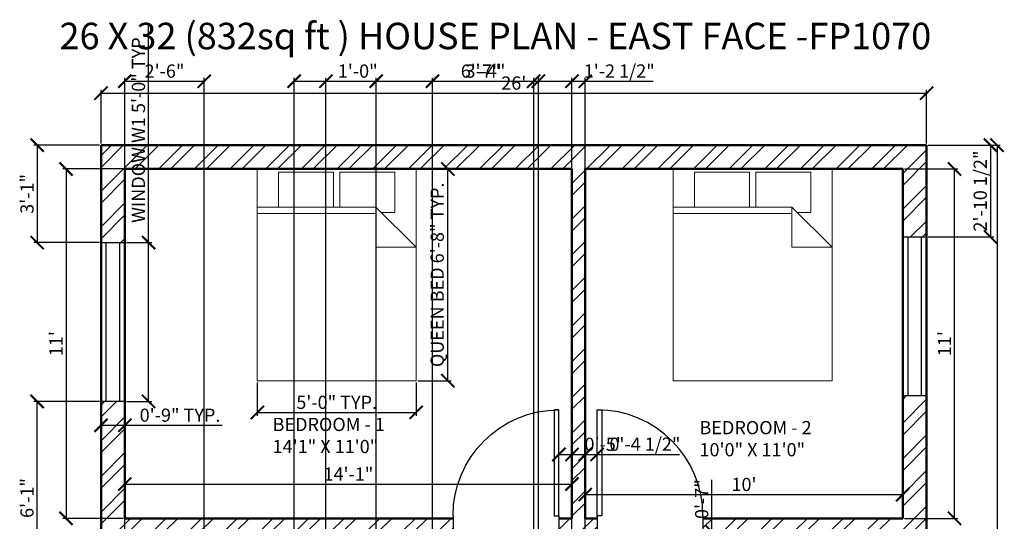
# Model space of a CAD drawing. Units: inches. Extents: x 683 to 1274, y 1901 to 2385.
# Tile 4 of 5: x 687 to 1059, y 2196 to 2385. Entities that reach past the tile are written whole.
import ezdxf

# ---------------------------------------------------------------- set-up
doc = ezdxf.new("R2010")
doc.units = ezdxf.units.IN
for name, color, linetype, lineweight in [('A-AREA-IDEN', 3, 'Continuous', 25), ('A-FURN', 2, 'Continuous', 18), ('A-WALL-PATT', 8, 'Continuous', 13), ('DIM', 3, 'Continuous', 18), ('DOORS', 4, 'Continuous', 25), ('TEXT', 1, 'Continuous', 25), ('walls', 6, 'Continuous', 50), ('WINDOWS', 30, 'Continuous', 25)]:
    doc.layers.add(name, color=color, linetype=linetype, lineweight=lineweight)
doc.styles.get("Standard").update_dxf_attribs({"font": 'arial.ttf'})
doc.dimstyles.new('ISO-25', dxfattribs={"dimtxt": 5, "dimasz": 5, "dimexe": 1.25, "dimexo": 0.625, "dimtad": 1, "dimdec": 1, "dimlunit": 4, "dimtxsty": 'Standard', "dimblk": 'ARCHTICK', "dimcen": 2.5, "dimadec": 0, "dimazin": 0, "dimtfac": 1, "dimtdec": 1, "dimtmove": 0, "dimatfit": 3, "dimfxl": 1, "dimarcsym": 0})

# ---------------------------------------------------------------- blocks, each defined once
blk = doc.blocks.new('Bed - Queen')
for p, q in [((0, -80.00003), (0, 0)), ((0, 0), (59.99999, 0)), ((59.99999, 0), (59.99999, -80.00003)), ((7.99999, -1.2), (28.79998, -1.2)), ((7.99999, -14.4), (7.99999, -1.2)), ((28.79998, -1.2), (28.79998, -14.4)), ((31.19999, -1.2), (51.99999, -1.2)), ((31.19999, -14.4), (31.19999, -1.2)), ((51.99999, -1.2), (51.99999, -16.4)), ((0, -14.4), (44.8, -14.4)), ((59.99999, -29.6), (44.8, -14.4)), ((44.8, -14.4), (44.8, -29.6)), ((44.8, -16.8), (0, -16.8)), ((51.99999, -16.4), (46.79936, -16.4)), ((44.8, -29.6), (59.99999, -29.6)), ((59.99999, -80.00003), (0, -80.00003))]:
    blk.add_line(p, q)
blk = doc.blocks.new('_ArchTick')
at = {"color": 0, "linetype": 'ByBlock', "const_width": 0.15}
blk.add_lwpolyline([(-0.5, -0.5), (0.5, 0.5)], dxfattribs=at)
blk = doc.blocks.new('*D6')
at = {"layer": 'Defpoints', "color": 0, "transparency": 16777216}
for p in [(1029.42, 2357.4), (717.42, 2337.78), (1029.42, 2337.78)]:
    blk.add_point(p, dxfattribs=at)
at = {"layer": 'DIM', "color": 0, "lineweight": -2, "transparency": 16777216}
for p, q in [((717.42, 2338.41), (717.42, 2358.65)), ((717.42, 2357.4), (1029.42, 2357.4)), ((1029.42, 2338.41), (1029.42, 2358.65))]:
    blk.add_line(p, q, dxfattribs=at)
at = {"layer": 'DIM', "color": 0, "lineweight": -2, "transparency": 16777216, "xscale": 5, "yscale": 5, "zscale": 5, "rotation": 180}
blk.add_blockref('_ArchTick', (717.42, 2357.4), dxfattribs=at)
at = {"layer": 'DIM', "color": 0, "lineweight": -2, "transparency": 16777216, "xscale": 5, "yscale": 5, "zscale": 5}
blk.add_blockref('_ArchTick', (1029.42, 2357.4), dxfattribs=at)
at = {"layer": 'DIM', "color": 0, "transparency": 16777216, "insert": (873.42, 2360.58), "char_height": 5, "attachment_point": 5}
blk.add_mtext("26'", dxfattribs=at)
blk = doc.blocks.new('*D7')
at = {"layer": 'Defpoints', "color": 0, "transparency": 16777216}
for p in [(1029.42, 2337.78), (1029.42, 1953.78), (1056.05, 1953.78)]:
    blk.add_point(p, dxfattribs=at)
at = {"layer": 'DIM', "color": 0, "lineweight": -2, "transparency": 16777216}
for p, q in [((1030.04, 2337.78), (1057.3, 2337.78)), ((1056.05, 2337.78), (1056.05, 1953.78)), ((1030.04, 1953.78), (1057.3, 1953.78))]:
    blk.add_line(p, q, dxfattribs=at)
at = {"layer": 'DIM', "color": 0, "lineweight": -2, "transparency": 16777216, "xscale": 5, "yscale": 5, "zscale": 5}
for p, rotation in [((1056.05, 2337.78), 90), ((1056.05, 1953.78), 270)]:
    blk.add_blockref('_ArchTick', p, dxfattribs=dict(at, rotation=rotation))
at = {"layer": 'DIM', "color": 0, "transparency": 16777216, "insert": (1052.87, 2145.78), "char_height": 5, "attachment_point": 5, "rotation": 90}
blk.add_mtext("32'", dxfattribs=at)
blk = doc.blocks.new('*D9')
at = {"layer": 'Defpoints', "color": 0, "transparency": 16777216}
for p in [(895.42, 2209.73), (726.42, 2196.78), (895.42, 2196.78)]:
    blk.add_point(p, dxfattribs=at)
at = {"layer": 'DIM', "color": 0, "lineweight": -2, "transparency": 16777216}
for p, q in [((726.42, 2197.41), (726.42, 2210.98)), ((895.42, 2197.41), (895.42, 2210.98)), ((726.42, 2209.73), (895.42, 2209.73))]:
    blk.add_line(p, q, dxfattribs=at)
at = {"layer": 'DIM', "color": 0, "lineweight": -2, "transparency": 16777216, "xscale": 5, "yscale": 5, "zscale": 5, "rotation": 180}
blk.add_blockref('_ArchTick', (726.42, 2209.73), dxfattribs=at)
at = {"layer": 'DIM', "color": 0, "lineweight": -2, "transparency": 16777216, "xscale": 5, "yscale": 5, "zscale": 5}
blk.add_blockref('_ArchTick', (895.42, 2209.73), dxfattribs=at)
at = {"layer": 'DIM', "color": 0, "transparency": 16777216, "insert": (810.92, 2212.86), "char_height": 5, "attachment_point": 5}
blk.add_mtext('14\'-1"', dxfattribs=at)
blk = doc.blocks.new('*D10')
at = {"layer": 'Defpoints', "color": 0, "transparency": 16777216}
for p in [(1020.42, 2205.76), (900.42, 2196.78), (1020.42, 2196.78)]:
    blk.add_point(p, dxfattribs=at)
at = {"layer": 'DIM', "color": 0, "lineweight": -2, "transparency": 16777216}
for p, q in [((900.42, 2197.41), (900.42, 2207.01)), ((1020.42, 2197.41), (1020.42, 2207.01)), ((900.42, 2205.76), (1020.42, 2205.76))]:
    blk.add_line(p, q, dxfattribs=at)
at = {"layer": 'DIM', "color": 0, "lineweight": -2, "transparency": 16777216, "xscale": 5, "yscale": 5, "zscale": 5, "rotation": 180}
blk.add_blockref('_ArchTick', (900.42, 2205.76), dxfattribs=at)
at = {"layer": 'DIM', "color": 0, "lineweight": -2, "transparency": 16777216, "xscale": 5, "yscale": 5, "zscale": 5}
blk.add_blockref('_ArchTick', (1020.42, 2205.76), dxfattribs=at)
at = {"layer": 'DIM', "color": 0, "transparency": 16777216, "insert": (960.42, 2208.94), "char_height": 5, "attachment_point": 5}
blk.add_mtext("10'", dxfattribs=at)
blk = doc.blocks.new('W1')
at = {"layer": 'WINDOWS'}
for p, q in [((1078.63, 2170.04), (1087.63, 2170.04)), ((1078.63, 2110.04), (1078.63, 2170.04)), ((1080.63, 2110.04), (1080.63, 2170.04)), ((1085.63, 2170.04), (1085.63, 2110.04)), ((1087.63, 2170.04), (1087.63, 2110.04)), ((1087.63, 2110.04), (1078.63, 2110.04))]:
    blk.add_line(p, q, dxfattribs=at)
blk = doc.blocks.new('*U18')
for p, q in [((0, 0), (0, -6)), ((40, 0), (40, -6))]:
    blk.add_line(p, q)
blk.add_lwpolyline([(0, 0), (0, 40), (1.75, 40), (1.75, 0)], close=True)
blk.add_arc((0, 0), 40, 0, 90)
blk = doc.blocks.new('*D19')
at = {"layer": 'Defpoints', "color": 0, "transparency": 16777216}
for p in [(726.42, 2328.78), (704.19, 2196.78), (726.42, 2196.78)]:
    blk.add_point(p, dxfattribs=at)
at = {"layer": 'DIM', "color": 0, "lineweight": -2, "transparency": 16777216}
for p, q in [((725.79, 2328.78), (702.94, 2328.78)), ((704.19, 2328.78), (704.19, 2196.78)), ((725.79, 2196.78), (702.94, 2196.78))]:
    blk.add_line(p, q, dxfattribs=at)
at = {"layer": 'DIM', "color": 0, "lineweight": -2, "transparency": 16777216, "xscale": 5, "yscale": 5, "zscale": 5}
for p, rotation in [((704.19, 2328.78), 90), ((704.19, 2196.78), 270)]:
    blk.add_blockref('_ArchTick', p, dxfattribs=dict(at, rotation=rotation))
at = {"layer": 'DIM', "color": 0, "transparency": 16777216, "insert": (701.05, 2262.78), "char_height": 5, "attachment_point": 5, "rotation": 90}
blk.add_mtext("11'", dxfattribs=at)
blk = doc.blocks.new('*D20')
at = {"layer": 'Defpoints', "color": 0, "transparency": 16777216}
for p in [(1020.42, 2328.78), (1040, 2328.78), (1020.42, 2196.78)]:
    blk.add_point(p, dxfattribs=at)
at = {"layer": 'DIM', "color": 0, "lineweight": -2, "transparency": 16777216}
for p, q in [((1021.04, 2328.78), (1041.25, 2328.78)), ((1040, 2196.78), (1040, 2328.78)), ((1021.04, 2196.78), (1041.25, 2196.78))]:
    blk.add_line(p, q, dxfattribs=at)
at = {"layer": 'DIM', "color": 0, "lineweight": -2, "transparency": 16777216, "xscale": 5, "yscale": 5, "zscale": 5}
for p, rotation in [((1040, 2328.78), 90), ((1040, 2196.78), 270)]:
    blk.add_blockref('_ArchTick', p, dxfattribs=dict(at, rotation=rotation))
at = {"layer": 'DIM', "color": 0, "transparency": 16777216, "insert": (1036.87, 2262.78), "char_height": 5, "attachment_point": 5, "rotation": 90}
blk.add_mtext("11'", dxfattribs=at)
blk = doc.blocks.new('*D25')
at = {"layer": 'Defpoints', "color": 0, "transparency": 16777216}
for p in [(836.49, 2328.78), (848.49, 2328.78), (836.49, 2248.78)]:
    blk.add_point(p, dxfattribs=at)
at = {"layer": 'DIM', "color": 0, "lineweight": -2, "transparency": 16777216}
for p, q in [((837.11, 2328.78), (849.74, 2328.78)), ((848.49, 2248.78), (848.49, 2328.78)), ((837.11, 2248.78), (849.74, 2248.78))]:
    blk.add_line(p, q, dxfattribs=at)
at = {"layer": 'DIM', "color": 0, "lineweight": -2, "transparency": 16777216, "xscale": 5, "yscale": 5, "zscale": 5}
for p, rotation in [((848.49, 2328.78), 90), ((848.49, 2248.78), 270)]:
    blk.add_blockref('_ArchTick', p, dxfattribs=dict(at, rotation=rotation))
at = {"layer": 'DIM', "color": 0, "transparency": 16777216, "insert": (845.12, 2288.78), "char_height": 5, "attachment_point": 5, "rotation": 90}
blk.add_mtext('QUEEN BED 6\'-8" TYP.', dxfattribs=at)
blk = doc.blocks.new('*D26')
at = {"layer": 'Defpoints', "color": 0, "transparency": 16777216}
for p in [(776.49, 2248.78), (836.49, 2248.78), (836.49, 2236.78)]:
    blk.add_point(p, dxfattribs=at)
at = {"layer": 'DIM', "color": 0, "lineweight": -2, "transparency": 16777216}
for p, q in [((776.49, 2248.16), (776.49, 2235.53)), ((836.49, 2248.16), (836.49, 2235.53)), ((776.49, 2236.78), (836.49, 2236.78))]:
    blk.add_line(p, q, dxfattribs=at)
at = {"layer": 'DIM', "color": 0, "lineweight": -2, "transparency": 16777216, "xscale": 5, "yscale": 5, "zscale": 5, "rotation": 180}
blk.add_blockref('_ArchTick', (776.49, 2236.78), dxfattribs=at)
at = {"layer": 'DIM', "color": 0, "lineweight": -2, "transparency": 16777216, "xscale": 5, "yscale": 5, "zscale": 5}
blk.add_blockref('_ArchTick', (836.49, 2236.78), dxfattribs=at)
at = {"layer": 'DIM', "color": 0, "transparency": 16777216, "insert": (806.49, 2239.96), "char_height": 5, "attachment_point": 5}
blk.add_mtext('5\'-0" TYP.', dxfattribs=at)
blk = doc.blocks.new('*D27')
at = {"layer": 'Defpoints', "color": 0, "transparency": 16777216}
for p in [(726.42, 2300.95), (735.42, 2300.95), (726.42, 2240.95)]:
    blk.add_point(p, dxfattribs=at)
at = {"layer": 'DIM', "color": 0, "lineweight": -2, "transparency": 16777216}
for p, q in [((735.42, 2300.95), (735.42, 2382.88)), ((727.04, 2300.95), (736.67, 2300.95)), ((735.42, 2240.95), (735.42, 2300.95)), ((727.04, 2240.95), (736.67, 2240.95))]:
    blk.add_line(p, q, dxfattribs=at)
at = {"layer": 'DIM', "color": 0, "lineweight": -2, "transparency": 16777216, "xscale": 5, "yscale": 5, "zscale": 5}
for p, rotation in [((735.42, 2300.95), 90), ((735.42, 2240.95), 270)]:
    blk.add_blockref('_ArchTick', p, dxfattribs=dict(at, rotation=rotation))
at = {"layer": 'DIM', "color": 0, "transparency": 16777216, "insert": (732.21, 2344.41), "char_height": 5, "attachment_point": 5, "rotation": 90}
blk.add_mtext('WINDOW W1 5\'-0" TYP.', dxfattribs=at)
blk = doc.blocks.new('*D28')
at = {"layer": 'Defpoints', "color": 0, "transparency": 16777216}
for p in [(717.42, 2240.95), (726.42, 2240.95), (726.42, 2231.95)]:
    blk.add_point(p, dxfattribs=at)
at = {"layer": 'DIM', "color": 0, "lineweight": -2, "transparency": 16777216}
for p, q in [((717.42, 2240.32), (717.42, 2230.7)), ((726.42, 2240.32), (726.42, 2230.7)), ((717.42, 2231.95), (726.42, 2231.95)), ((726.42, 2231.95), (763.15, 2231.95))]:
    blk.add_line(p, q, dxfattribs=at)
at = {"layer": 'DIM', "color": 0, "lineweight": -2, "transparency": 16777216, "xscale": 5, "yscale": 5, "zscale": 5, "rotation": 180}
blk.add_blockref('_ArchTick', (717.42, 2231.95), dxfattribs=at)
at = {"layer": 'DIM', "color": 0, "lineweight": -2, "transparency": 16777216, "xscale": 5, "yscale": 5, "zscale": 5}
blk.add_blockref('_ArchTick', (726.42, 2231.95), dxfattribs=at)
at = {"layer": 'DIM', "color": 0, "transparency": 16777216, "insert": (747.28, 2235.12), "char_height": 5, "attachment_point": 5}
blk.add_mtext('0\'-9" TYP.', dxfattribs=at)
blk = doc.blocks.new('*D39')
at = {"layer": 'Defpoints', "color": 0, "transparency": 16777216}
for p in [(900.42, 2361.93), (821.42, 1929.78), (900.42, 1929.78)]:
    blk.add_point(p, dxfattribs=at)
at = {"layer": 'DIM', "color": 0, "lineweight": -2, "transparency": 16777216}
for p, q in [((821.42, 1930.41), (821.42, 2363.18)), ((900.42, 1930.41), (900.42, 2363.18)), ((821.42, 2361.93), (900.42, 2361.93))]:
    blk.add_line(p, q, dxfattribs=at)
at = {"layer": 'DIM', "color": 0, "lineweight": -2, "transparency": 16777216, "xscale": 5, "yscale": 5, "zscale": 5, "rotation": 180}
blk.add_blockref('_ArchTick', (821.42, 2361.93), dxfattribs=at)
at = {"layer": 'DIM', "color": 0, "lineweight": -2, "transparency": 16777216, "xscale": 5, "yscale": 5, "zscale": 5}
blk.add_blockref('_ArchTick', (900.42, 2361.93), dxfattribs=at)
at = {"layer": 'DIM', "color": 0, "transparency": 16777216, "insert": (860.92, 2365.11), "char_height": 5, "attachment_point": 5}
blk.add_mtext('6\'-7"', dxfattribs=at)
blk = doc.blocks.new('*D44')
at = {"layer": 'Defpoints', "color": 0, "transparency": 16777216}
for p in [(882.7, 2361.93), (842.7, 1953.78), (882.7, 1953.78)]:
    blk.add_point(p, dxfattribs=at)
at = {"layer": 'DIM', "color": 0, "lineweight": -2, "transparency": 16777216}
for p, q in [((842.7, 1954.41), (842.7, 2363.18)), ((882.7, 1954.41), (882.7, 2363.18)), ((842.7, 2361.93), (882.7, 2361.93))]:
    blk.add_line(p, q, dxfattribs=at)
at = {"layer": 'DIM', "color": 0, "lineweight": -2, "transparency": 16777216, "xscale": 5, "yscale": 5, "zscale": 5, "rotation": 180}
blk.add_blockref('_ArchTick', (842.7, 2361.93), dxfattribs=at)
at = {"layer": 'DIM', "color": 0, "lineweight": -2, "transparency": 16777216, "xscale": 5, "yscale": 5, "zscale": 5}
blk.add_blockref('_ArchTick', (882.7, 2361.93), dxfattribs=at)
at = {"layer": 'DIM', "color": 0, "transparency": 16777216, "insert": (862.7, 2365.11), "char_height": 5, "attachment_point": 5}
blk.add_mtext('3\'-4"', dxfattribs=at)
blk = doc.blocks.new('*D50')
at = {"layer": 'Defpoints', "color": 0, "transparency": 16777216}
for p in [(802.42, 2361.93), (790.42, 2085.78), (802.42, 2085.78)]:
    blk.add_point(p, dxfattribs=at)
at = {"layer": 'DIM', "color": 0, "lineweight": -2, "transparency": 16777216}
for p, q in [((790.42, 2086.41), (790.42, 2363.18)), ((802.42, 2086.41), (802.42, 2363.18)), ((790.42, 2361.93), (802.42, 2361.93)), ((802.42, 2361.93), (821.49, 2361.93))]:
    blk.add_line(p, q, dxfattribs=at)
at = {"layer": 'DIM', "color": 0, "lineweight": -2, "transparency": 16777216, "xscale": 5, "yscale": 5, "zscale": 5, "rotation": 180}
blk.add_blockref('_ArchTick', (790.42, 2361.93), dxfattribs=at)
at = {"layer": 'DIM', "color": 0, "lineweight": -2, "transparency": 16777216, "xscale": 5, "yscale": 5, "zscale": 5}
blk.add_blockref('_ArchTick', (802.42, 2361.93), dxfattribs=at)
at = {"layer": 'DIM', "color": 0, "transparency": 16777216, "insert": (814.45, 2365.11), "char_height": 5, "attachment_point": 5}
blk.add_mtext('1\'-0"', dxfattribs=at)
blk = doc.blocks.new('*D51')
at = {"layer": 'Defpoints', "color": 0, "transparency": 16777216}
for p in [(717.42, 2337.78), (693.27, 2300.95), (717.42, 2300.95)]:
    blk.add_point(p, dxfattribs=at)
at = {"layer": 'DIM', "color": 0, "lineweight": -2, "transparency": 16777216}
for p, q in [((716.79, 2337.78), (692.02, 2337.78)), ((693.27, 2337.78), (693.27, 2300.95)), ((716.79, 2300.95), (692.02, 2300.95))]:
    blk.add_line(p, q, dxfattribs=at)
at = {"layer": 'DIM', "color": 0, "lineweight": -2, "transparency": 16777216, "xscale": 5, "yscale": 5, "zscale": 5}
for p, rotation in [((693.27, 2337.78), 90), ((693.27, 2300.95), 270)]:
    blk.add_blockref('_ArchTick', p, dxfattribs=dict(at, rotation=rotation))
at = {"layer": 'DIM', "color": 0, "transparency": 16777216, "insert": (690.09, 2319.36), "char_height": 5, "attachment_point": 5, "rotation": 90}
blk.add_mtext('3\'-1"', dxfattribs=at)
blk = doc.blocks.new('*D52')
at = {"layer": 'Defpoints', "color": 0, "transparency": 16777216}
for p in [(1029.42, 2337.78), (1029.42, 2303.09), (1053.57, 2303.09)]:
    blk.add_point(p, dxfattribs=at)
at = {"layer": 'DIM', "color": 0, "lineweight": -2, "transparency": 16777216}
for p, q in [((1030.04, 2337.78), (1054.82, 2337.78)), ((1053.57, 2337.78), (1053.57, 2303.09)), ((1030.04, 2303.09), (1054.82, 2303.09))]:
    blk.add_line(p, q, dxfattribs=at)
at = {"layer": 'DIM', "color": 0, "lineweight": -2, "transparency": 16777216, "xscale": 5, "yscale": 5, "zscale": 5}
for p, rotation in [((1053.57, 2337.78), 90), ((1053.57, 2303.09), 270)]:
    blk.add_blockref('_ArchTick', p, dxfattribs=dict(at, rotation=rotation))
at = {"layer": 'DIM', "color": 0, "transparency": 16777216, "insert": (1050.36, 2320.44), "char_height": 5, "attachment_point": 5, "rotation": 90}
blk.add_mtext('2\'-10 1/2"', dxfattribs=at)
blk = doc.blocks.new('*D55')
at = {"layer": 'Defpoints', "color": 0, "transparency": 16777216}
for p in [(693.27, 2240.95), (717.42, 2240.95), (717.42, 2167.98)]:
    blk.add_point(p, dxfattribs=at)
at = {"layer": 'DIM', "color": 0, "lineweight": -2, "transparency": 16777216}
for p, q in [((716.79, 2240.95), (692.02, 2240.95)), ((693.27, 2167.98), (693.27, 2240.95)), ((716.79, 2167.98), (692.02, 2167.98))]:
    blk.add_line(p, q, dxfattribs=at)
at = {"layer": 'DIM', "color": 0, "lineweight": -2, "transparency": 16777216, "xscale": 5, "yscale": 5, "zscale": 5}
for p, rotation in [((693.27, 2240.95), 90), ((693.27, 2167.98), 270)]:
    blk.add_blockref('_ArchTick', p, dxfattribs=dict(at, rotation=rotation))
at = {"layer": 'DIM', "color": 0, "transparency": 16777216, "insert": (690.09, 2204.46), "char_height": 5, "attachment_point": 5, "rotation": 90}
blk.add_mtext('6\'-1"', dxfattribs=at)
blk = doc.blocks.new('*D58')
at = {"layer": 'Defpoints', "color": 0, "transparency": 16777216}
for p in [(756.42, 2361.93), (726.42, 2044.78), (756.42, 2044.78)]:
    blk.add_point(p, dxfattribs=at)
at = {"layer": 'DIM', "color": 0, "lineweight": -2, "transparency": 16777216}
for p, q in [((726.42, 2045.41), (726.42, 2363.18)), ((756.42, 2045.41), (756.42, 2363.18)), ((726.42, 2361.93), (756.42, 2361.93))]:
    blk.add_line(p, q, dxfattribs=at)
at = {"layer": 'DIM', "color": 0, "lineweight": -2, "transparency": 16777216, "xscale": 5, "yscale": 5, "zscale": 5, "rotation": 180}
blk.add_blockref('_ArchTick', (726.42, 2361.93), dxfattribs=at)
at = {"layer": 'DIM', "color": 0, "lineweight": -2, "transparency": 16777216, "xscale": 5, "yscale": 5, "zscale": 5}
blk.add_blockref('_ArchTick', (756.42, 2361.93), dxfattribs=at)
at = {"layer": 'DIM', "color": 0, "transparency": 16777216, "insert": (741.42, 2365.11), "char_height": 5, "attachment_point": 5}
blk.add_mtext('2\'-6"', dxfattribs=at)
blk = doc.blocks.new('*D61')
at = {"layer": 'Defpoints', "color": 0, "transparency": 16777216}
for p in [(895.42, 2361.93), (880.95, 1962.78), (895.42, 1962.78)]:
    blk.add_point(p, dxfattribs=at)
at = {"layer": 'DIM', "color": 0, "lineweight": -2, "transparency": 16777216}
for p, q in [((880.95, 1963.41), (880.95, 2363.18)), ((895.42, 1963.41), (895.42, 2363.18)), ((880.95, 2361.93), (895.42, 2361.93)), ((895.42, 2361.93), (926.14, 2361.93))]:
    blk.add_line(p, q, dxfattribs=at)
at = {"layer": 'DIM', "color": 0, "lineweight": -2, "transparency": 16777216, "xscale": 5, "yscale": 5, "zscale": 5, "rotation": 180}
blk.add_blockref('_ArchTick', (880.95, 2361.93), dxfattribs=at)
at = {"layer": 'DIM', "color": 0, "lineweight": -2, "transparency": 16777216, "xscale": 5, "yscale": 5, "zscale": 5}
blk.add_blockref('_ArchTick', (895.42, 2361.93), dxfattribs=at)
at = {"layer": 'DIM', "color": 0, "transparency": 16777216, "insert": (913.28, 2365.14), "char_height": 5, "attachment_point": 5}
blk.add_mtext('1\'-2 1/2"', dxfattribs=at)
blk = doc.blocks.new('*D63')
at = {"layer": 'Defpoints', "color": 0, "transparency": 16777216}
for p in [(895.42, 2220.93), (890.48, 2196.78), (895.42, 2196.78)]:
    blk.add_point(p, dxfattribs=at)
at = {"layer": 'DIM', "color": 0, "lineweight": -2, "transparency": 16777216}
for p, q in [((890.48, 2197.41), (890.48, 2222.18)), ((895.42, 2197.41), (895.42, 2222.18)), ((890.48, 2220.93), (895.42, 2220.93)), ((895.42, 2220.93), (914.96, 2220.93))]:
    blk.add_line(p, q, dxfattribs=at)
at = {"layer": 'DIM', "color": 0, "lineweight": -2, "transparency": 16777216, "xscale": 5, "yscale": 5, "zscale": 5, "rotation": 180}
blk.add_blockref('_ArchTick', (890.48, 2220.93), dxfattribs=at)
at = {"layer": 'DIM', "color": 0, "lineweight": -2, "transparency": 16777216, "xscale": 5, "yscale": 5, "zscale": 5}
blk.add_blockref('_ArchTick', (895.42, 2220.93), dxfattribs=at)
at = {"layer": 'DIM', "color": 0, "transparency": 16777216, "insert": (907.69, 2224.11), "char_height": 5, "attachment_point": 5}
blk.add_mtext('0\'-5"', dxfattribs=at)
blk = doc.blocks.new('*D64')
at = {"layer": 'Defpoints', "color": 0, "transparency": 16777216}
for p in [(904.89, 2220.93), (900.42, 2196.78), (904.89, 2196.78)]:
    blk.add_point(p, dxfattribs=at)
at = {"layer": 'DIM', "color": 0, "lineweight": -2, "transparency": 16777216}
for p, q in [((900.42, 2197.41), (900.42, 2222.18)), ((904.89, 2197.41), (904.89, 2222.18)), ((900.42, 2220.93), (904.89, 2220.93)), ((904.89, 2220.93), (936.09, 2220.93))]:
    blk.add_line(p, q, dxfattribs=at)
at = {"layer": 'DIM', "color": 0, "lineweight": -2, "transparency": 16777216, "xscale": 5, "yscale": 5, "zscale": 5, "rotation": 180}
blk.add_blockref('_ArchTick', (900.42, 2220.93), dxfattribs=at)
at = {"layer": 'DIM', "color": 0, "lineweight": -2, "transparency": 16777216, "xscale": 5, "yscale": 5, "zscale": 5}
blk.add_blockref('_ArchTick', (904.89, 2220.93), dxfattribs=at)
at = {"layer": 'DIM', "color": 0, "transparency": 16777216, "insert": (922.99, 2224.14), "char_height": 5, "attachment_point": 5}
blk.add_mtext('0\'-4 1/2"', dxfattribs=at)
blk = doc.blocks.new('*D67')
at = {"layer": 'Defpoints', "color": 0, "transparency": 16777216}
for p in [(948.27, 2191.78), (972.42, 2191.78), (972.42, 2184.95)]:
    blk.add_point(p, dxfattribs=at)
at = {"layer": 'DIM', "color": 0, "lineweight": -2, "transparency": 16777216}
for p, q in [((948.27, 2191.78), (948.27, 2211.32)), ((971.79, 2191.78), (947.02, 2191.78)), ((948.27, 2184.95), (948.27, 2191.78)), ((971.79, 2184.95), (947.02, 2184.95))]:
    blk.add_line(p, q, dxfattribs=at)
at = {"layer": 'DIM', "color": 0, "lineweight": -2, "transparency": 16777216, "xscale": 5, "yscale": 5, "zscale": 5}
for p, rotation in [((948.27, 2191.78), 90), ((948.27, 2184.95), 270)]:
    blk.add_blockref('_ArchTick', p, dxfattribs=dict(at, rotation=rotation))
at = {"layer": 'DIM', "color": 0, "transparency": 16777216, "insert": (945.09, 2204.05), "char_height": 5, "attachment_point": 5, "rotation": 90}
blk.add_mtext('0\'-7"', dxfattribs=at)

msp = doc.modelspace()

# ---------------------------------------------------------------- hatches: boundary and pattern name
at = {"layer": 'A-WALL-PATT'}
h = msp.add_hatch(dxfattribs=at)
h.set_pattern_fill('ANSI32', color=256)
h.paths.add_polyline_path([(717.42, 2337.78), (717.42, 2300.95), (726.42, 2300.95), (726.42, 2328.78), (895.42, 2328.78), (895.42, 2196.78), (890.48, 2196.78), (890.48, 2191.78), (904.89, 2191.78), (904.89, 2196.78), (900.42, 2196.78), (900.42, 2328.78), (1020.42, 2328.78), (1020.42, 2303.09), (1029.42, 2303.09), (1029.42, 2337.78)])
h.paths.add_polyline_path([(1020.42, 2196.78), (944.89, 2196.78), (944.89, 2191.78), (967.42, 2191.78), (967.42, 2184.95), (972.42, 2184.95), (972.42, 2191.78), (1020.42, 2191.78), (1020.42, 2129.51), (1029.42, 2129.51), (1029.42, 2243.09), (1020.42, 2243.09)])
h.paths.add_polyline_path([(1029.42, 2105.51), (1020.42, 2105.51), (1020.42, 2100.78), (972.42, 2100.78), (972.42, 2150.14), (967.42, 2150.14), (967.42, 2100.78), (895.42, 2100.78), (895.42, 2088.36), (900.42, 2088.36), (900.42, 2095.78), (1020.42, 2095.78), (1020.42, 1962.78), (1000.32, 1962.78), (1000.32, 1953.78), (1029.42, 1953.78)])
h.paths.add_polyline_path([(940.32, 1953.78), (940.32, 1962.78), (900.42, 1962.78), (900.42, 2048.36), (895.42, 2048.36), (895.42, 1962.78), (882.7, 1962.78), (882.7, 1959.78), (882.7, 1953.78)])
h.paths.add_polyline_path([(790.86, 1953.78), (790.86, 1962.78), (726.42, 1962.78), (726.42, 1980.18), (717.42, 1980.18), (717.42, 1953.78)])
h.paths.add_polyline_path([(842.7, 1953.78), (842.7, 1959.78, -0.01877), (842.81, 1962.78), (826.42, 1962.78), (826.42, 2003.23), (821.42, 2003.23), (821.42, 1962.78), (814.86, 1962.78), (814.86, 1953.78)])
h.paths.add_polyline_path([(726.42, 2196.78), (726.42, 2240.95), (717.42, 2240.95), (717.42, 2167.98), (726.42, 2167.98), (726.42, 2191.78), (850.48, 2191.78), (850.48, 2196.78)])

# ---------------------------------------------------------------- linework, layer by layer
at = {"layer": 'walls'}
for p, q in [((717.42, 2337.78), (1029.42, 2337.78)), ((717.42, 2337.78), (717.42, 1953.78)), ((1029.42, 2337.78), (1029.42, 1953.78)), ((726.42, 2328.78), (895.42, 2328.78)), ((726.42, 2328.78), (726.42, 2196.78)), ((895.42, 2328.78), (895.42, 2196.78)), ((900.42, 2328.78), (900.42, 2196.78)), ((900.42, 2328.78), (1020.42, 2328.78)), ((1020.42, 2328.78), (1020.42, 2196.78)), ((726.42, 2196.78), (850.48, 2196.78)), ((890.48, 2196.78), (895.42, 2196.78)), ((900.42, 2196.78), (904.89, 2196.78)), ((944.89, 2196.78), (1020.42, 2196.78))]:
    msp.add_line(p, q, dxfattribs=at)

# ---------------------------------------------------------------- block references
at = {"layer": 'A-FURN'}
for p in [(776.49, 2328.78), (933.7, 2328.78)]:
    msp.add_blockref('Bed - Queen', p, dxfattribs=at)
at = {"layer": 'DOORS', "xscale": -1}
msp.add_blockref('*U18', (890.48, 2197.78), dxfattribs=at)
at = {"layer": 'DOORS'}
msp.add_blockref('*U18', (904.89, 2197.78), dxfattribs=at)
at = {"layer": 'WINDOWS'}
for p in [(-361.21, 130.9), (-58.21, 133.05)]:
    msp.add_blockref('W1', p, dxfattribs=at)

# ---------------------------------------------------------------- texts
at = {"layer": 'A-AREA-IDEN', "char_height": 5, "attachment_point": 1}
for s, width, insert in [('{BEDROOM - 1 \\P14\'1" X 11\'0"}', 67.9765, (782.27, 2234.75)), ('{BEDROOM - 2 \\P10\'0" X 11\'0"}', 48.7562, (943.6, 2233.55))]:
    msp.add_mtext_dynamic_manual_height_columns(s, width=width, gutter_width=12.5, heights=[0], dxfattribs=dict(at, insert=insert))
at = {"layer": 'TEXT', "insert": (701.73, 2384.01), "char_height": 10, "attachment_point": 1}
msp.add_mtext_dynamic_manual_height_columns('26 X 32 (832sq ft ) HOUSE PLAN - EAST FACE -FP1070', width=362.0519, gutter_width=12.5, heights=[0], dxfattribs=at)

# ---------------------------------------------------------------- dimensions: what is measured, and where the dimension line sits
at = {"layer": 'DIM'}
for base, p1, p2, text, picture, middle in [((735.42, 2300.95), (726.42, 2240.95), (726.42, 2300.95), 'WINDOW W1 <> TYP.', '*D27', (732.21, 2344.41)), ((848.49, 2328.78), (836.49, 2248.78), (836.49, 2328.78), 'QUEEN BED <> TYP.', '*D25', (845.12, 2288.78))]:
    dim = msp.add_linear_dim(base=base, p1=p1, p2=p2, angle=90, text=text, dimstyle='ISO-25', override={"dimdec": 1, "dimlfac": 1, "dimrnd": 0, "dimzin": 1, "dimdsep": 46, "dimlunit": 4, "dimfrac": 2}, dxfattribs=at)
    dim.commit()
    dim.dimension.update_dxf_attribs({"geometry": picture, "text_midpoint": middle})
for base, p1, p2, override, picture, middle in [((895.42, 2361.93), (880.95, 1962.78), (895.42, 1962.78), {"dimdec": 1, "dimlfac": 1, "dimrnd": 0, "dimzin": 1, "dimdsep": 46, "dimlunit": 4, "dimfrac": 2}, '*D61', (913.28, 2365.14)), ((756.42, 2361.93), (726.42, 2044.78), (756.42, 2044.78), {"dimdec": 1, "dimlfac": 1, "dimrnd": 0, "dimzin": 1, "dimdsep": 46, "dimlunit": 4, "dimfrac": 2}, '*D58', (741.42, 2365.11)), ((802.42, 2361.93), (790.42, 2085.78), (802.42, 2085.78), {"dimdec": 1, "dimlfac": 1, "dimrnd": 0, "dimzin": 1, "dimdsep": 46, "dimlunit": 4, "dimfrac": 2}, '*D50', (814.45, 2365.11)), ((900.42, 2361.93), (821.42, 1929.78), (900.42, 1929.78), {"dimdec": 1, "dimlfac": 1, "dimrnd": 0, "dimzin": 1, "dimdsep": 46, "dimlunit": 4, "dimfrac": 2}, '*D39', (860.92, 2365.11)), ((882.7, 2361.93), (842.7, 1953.78), (882.7, 1953.78), {"dimdec": 1, "dimlfac": 1, "dimrnd": 0, "dimzin": 1, "dimdsep": 46, "dimlunit": 4, "dimfrac": 2}, '*D44', (862.7, 2365.11)), ((1029.42, 2357.4), (717.42, 2337.78), (1029.42, 2337.78), {"dimclrd": 0, "dimclre": 0, "dimclrt": 0}, '*D6', (873.42, 2360.58)), ((904.89, 2220.93), (900.42, 2196.78), (904.89, 2196.78), {"dimdec": 1, "dimlfac": 1, "dimrnd": 0, "dimzin": 1, "dimdsep": 46, "dimlunit": 4, "dimfrac": 2}, '*D64', (922.99, 2224.14)), ((895.42, 2220.93), (890.48, 2196.78), (895.42, 2196.78), {"dimdec": 1, "dimlfac": 1, "dimrnd": 0, "dimzin": 1, "dimdsep": 46, "dimlunit": 4, "dimfrac": 2}, '*D63', (907.69, 2224.11)), ((895.42, 2209.73), (726.42, 2196.78), (895.42, 2196.78), {"dimclrd": 0, "dimclre": 0, "dimclrt": 0}, '*D9', (810.92, 2212.86)), ((1020.42, 2205.76), (900.42, 2196.78), (1020.42, 2196.78), {"dimclrd": 0, "dimclre": 0, "dimclrt": 0}, '*D10', (960.42, 2208.94))]:
    dim = msp.add_linear_dim(base=base, p1=p1, p2=p2, dimstyle='ISO-25', override=override, dxfattribs=at)
    dim.commit()
    dim.dimension.update_dxf_attribs({"geometry": picture, "text_midpoint": middle})
for base, p1, p2, override, picture, middle in [((693.27, 2300.95), (717.42, 2337.78), (717.42, 2300.95), {"dimdec": 1, "dimlfac": 1, "dimrnd": 0, "dimzin": 1, "dimdsep": 46, "dimlunit": 4, "dimfrac": 2}, '*D51', (690.09, 2319.36)), ((1056.05, 1953.78), (1029.42, 2337.78), (1029.42, 1953.78), {"dimclrd": 0, "dimclre": 0, "dimclrt": 0}, '*D7', (1052.87, 2145.78)), ((1053.57, 2303.09), (1029.42, 2337.78), (1029.42, 2303.09), {"dimdec": 1, "dimlfac": 1, "dimrnd": 0, "dimzin": 1, "dimdsep": 46, "dimlunit": 4, "dimfrac": 2}, '*D52', (1050.36, 2320.44)), ((704.19, 2196.78), (726.42, 2328.78), (726.42, 2196.78), {"dimclrd": 0, "dimclre": 0, "dimclrt": 0}, '*D19', (701.05, 2262.78)), ((1040, 2328.78), (1020.42, 2196.78), (1020.42, 2328.78), {"dimclrd": 0, "dimclre": 0, "dimclrt": 0}, '*D20', (1036.87, 2262.78)), ((693.27, 2240.95), (717.42, 2167.98), (717.42, 2240.95), {"dimdec": 1, "dimlfac": 1, "dimrnd": 0, "dimzin": 1, "dimdsep": 46, "dimlunit": 4, "dimfrac": 2}, '*D55', (690.09, 2204.46)), ((948.27, 2191.78), (972.42, 2184.95), (972.42, 2191.78), {"dimdec": 1, "dimlfac": 1, "dimrnd": 0, "dimzin": 1, "dimdsep": 46, "dimlunit": 4, "dimfrac": 2}, '*D67', (945.09, 2204.05))]:
    dim = msp.add_linear_dim(base=base, p1=p1, p2=p2, angle=90, dimstyle='ISO-25', override=override, dxfattribs=at)
    dim.commit()
    dim.dimension.update_dxf_attribs({"geometry": picture, "text_midpoint": middle})
for base, p1, p2, picture, middle in [((836.49, 2236.78), (776.49, 2248.78), (836.49, 2248.78), '*D26', (806.49, 2239.96)), ((726.42, 2231.95), (717.42, 2240.95), (726.42, 2240.95), '*D28', (747.28, 2235.12))]:
    dim = msp.add_linear_dim(base=base, p1=p1, p2=p2, text='<> TYP.', dimstyle='ISO-25', override={"dimdec": 1, "dimlfac": 1, "dimrnd": 0, "dimzin": 1, "dimdsep": 46, "dimlunit": 4, "dimfrac": 2}, dxfattribs=at)
    dim.commit()
    dim.dimension.update_dxf_attribs({"geometry": picture, "text_midpoint": middle})

doc.saveas('drawing.dxf')
